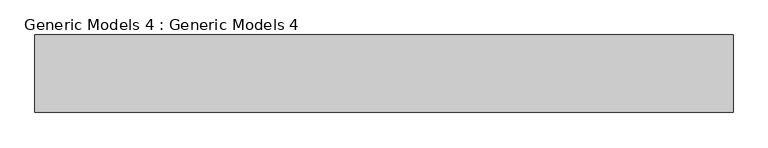
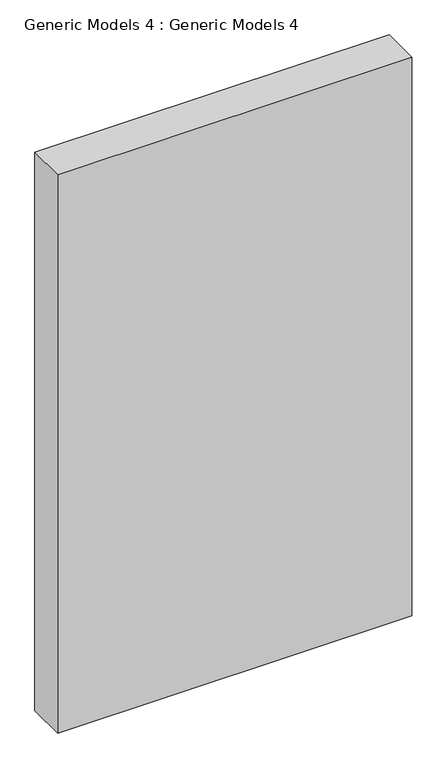
"""IFC4 building model written with IfcOpenShell, lengths in millimetres: proxy geometry, Generic Models 4 : Generic Models 4."""

from ifc_helpers import new_model, si_unit, origin, origin_with_axes, place, context, project, spatial, polyline, outline, extrude, source, transform, mapped, element, save


def generic_models_4_generic_models_4_91b2e968(model_context):
    return source(origin(), model_context, "Body", "SweptSolid", [
        extrude(outline(polyline([(2418.354407, -3908.274389), (2418.354407, -4111.474389), (589.554407, -4111.474389), (589.554407, -3908.274389), (2418.354407, -3908.274389)])), origin_with_axes(), (0.0, 0.0, 1.0), 3048.0),
    ])


if __name__ == "__main__":
    model = new_model("IFC4")
    model_context = context("Model", 3, world=origin())
    ifc_project = project(units=[si_unit("LENGTHUNIT", "METRE", prefix="MILLI")], contexts=[model_context])
    site = spatial("IfcSite", under=ifc_project)
    building = spatial("IfcBuilding", under=site)
    placement = place(None, origin())
    generic_models_4_generic_models_4_shape = generic_models_4_generic_models_4_91b2e968(model_context)
    element("IfcBuildingElementProxy", 1, Name="Generic Models 4 : Generic Models 4", ObjectType="Generic Models 4 : Generic Models 4", at=placement, inside=building, context=model_context, shape_type="MappedRepresentation", body=[
        mapped(generic_models_4_generic_models_4_shape, transform((0.0, 0.0, 0.0), x_axis=(1.0, 0.0, 0.0), y_axis=(0.0, 1.0, 0.0), z_axis=(0.0, 0.0, 1.0))),
    ])
    save(model, "model.ifc")

# Revit data of these elements
# Element 1 (IfcBuildingElementProxy, "Generic Models 4 : Generic Models 4")
#   Materials on its faces: "Asphalt Shingle"
# Materials
#   "Asphalt Shingle": class "Generic", colour RGB 155 155 155, transparency 0, Description = "Asphalt roofing shingle", Cost = 0
